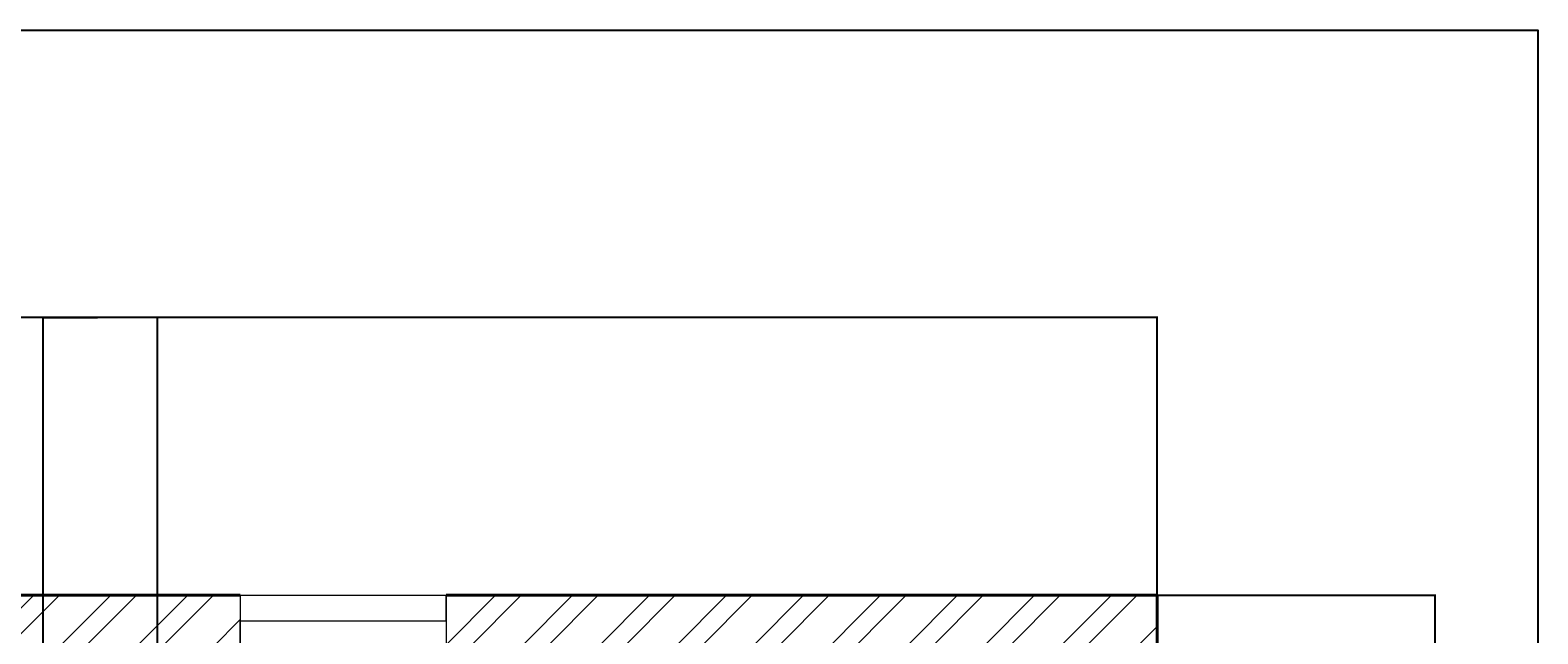
# Model space of a CAD drawing. Units: inches. Extents: x 1601 to 2297, y 1496 to 2631.
# Tile 57 of 57: x 2033 to 2297, y 2526 to 2631. Entities that reach past the tile are written whole.
import ezdxf

# ---------------------------------------------------------------- set-up
doc = ezdxf.new("R2010")
doc.units = ezdxf.units.IN
for name, color, linetype, lineweight in [('A-ANNO-DIMS', 2, 'Continuous', 18), ('A-ANNO-TTLB', 7, 'Continuous', 25), ('A-GLAZ', 161, 'Continuous', 20), ('A-WALL', 7, 'Continuous', 40), ('A-WALL-PATT', 215, 'Continuous', 13)]:
    doc.layers.add(name, color=color, linetype=linetype, lineweight=lineweight)
doc.styles.get("Standard").update_dxf_attribs({"font": 'arial.ttf'})
doc.dimstyles.get("Standard").update_dxf_attribs({"dimtxt": 0.18, "dimasz": 0.18, "dimexe": 0.18, "dimexo": 0.0625, "dimgap": 0.09, "dimtad": 0, "dimtih": 1, "dimtoh": 1, "dimdec": 4, "dimzin": 0, "dimdsep": 46, "dimtxsty": 'Standard', "dimcen": 0.09, "dimadec": 0, "dimazin": 0, "dimtfac": 1, "dimtdec": 4, "dimtofl": 0, "dimtmove": 0, "dimatfit": 3, "dimfxl": 1, "dimtolj": 1, "dimtzin": 0, "dimarcsym": 0})

# ---------------------------------------------------------------- blocks, each defined once
blk = doc.blocks.new('*D28')
at = {"layer": 'A-ANNO-DIMS', "color": 0, "lineweight": -2, "transparency": 16777216}
for p, q in [((1686.04, 2532.39), (1686.04, 2581.06)), ((1686.22, 2580.88), (1957.89, 2580.88)), ((2230.36, 2580.88), (1958.68, 2580.88)), ((2230.54, 2532.39), (2230.54, 2581.06))]:
    blk.add_line(p, q, dxfattribs=at)
at = {"layer": 'A-ANNO-DIMS', "color": 0, "transparency": 16777216}
for points in [[(1686.22, 2580.91), (1686.22, 2580.85), (1686.04, 2580.88)], [(2230.36, 2580.91), (2230.36, 2580.85), (2230.54, 2580.88)]]:
    blk.add_solid(points, dxfattribs=at)
at = {"layer": 'Defpoints', "color": 0, "transparency": 16777216}
for p in [(2230.54, 2580.88), (1686.04, 2532.33), (2230.54, 2532.33)]:
    blk.add_point(p, dxfattribs=at)
at = {"layer": 'A-ANNO-DIMS', "color": 0, "transparency": 16777216, "insert": (1958.29, 2580.88), "char_height": 0.18, "attachment_point": 5}
blk.add_mtext('\\A1;544.5', dxfattribs=at)
blk = doc.blocks.new('*D29')
at = {"layer": 'A-ANNO-DIMS', "color": 0, "lineweight": -2, "transparency": 16777216}
for p, q in [((2230.6, 2532.33), (2279.27, 2532.33)), ((2279.09, 2532.15), (2279.09, 2084.01)), ((2279.09, 1635.51), (2279.09, 2083.64)), ((2230.6, 1635.33), (2279.27, 1635.33))]:
    blk.add_line(p, q, dxfattribs=at)
at = {"layer": 'A-ANNO-DIMS', "color": 0, "transparency": 16777216}
for points in [[(2279.06, 2532.15), (2279.12, 2532.15), (2279.09, 2532.33)], [(2279.06, 1635.51), (2279.12, 1635.51), (2279.09, 1635.33)]]:
    blk.add_solid(points, dxfattribs=at)
at = {"layer": 'Defpoints', "color": 0, "transparency": 16777216}
for p in [(2230.54, 2532.33), (2279.09, 2532.33), (2230.54, 1635.33)]:
    blk.add_point(p, dxfattribs=at)
at = {"layer": 'A-ANNO-DIMS', "color": 0, "transparency": 16777216, "insert": (2279.09, 2083.83), "char_height": 0.18, "attachment_point": 5}
blk.add_mtext('\\A1;897', dxfattribs=at)
blk = doc.blocks.new('*D40')
at = {"layer": 'A-ANNO-DIMS', "color": 0, "lineweight": -2, "transparency": 16777216}
for p, q in [((2035.54, 1986.39), (2035.54, 2581.06)), ((2035.72, 2580.88), (2045.08, 2580.88)), ((2055.37, 2580.88), (2046.01, 2580.88)), ((2055.55, 1986.39), (2055.55, 2581.06))]:
    blk.add_line(p, q, dxfattribs=at)
at = {"layer": 'A-ANNO-DIMS', "color": 0, "transparency": 16777216}
for points in [[(2035.72, 2580.91), (2035.72, 2580.85), (2035.54, 2580.88)], [(2055.37, 2580.91), (2055.37, 2580.85), (2055.55, 2580.88)]]:
    blk.add_solid(points, dxfattribs=at)
at = {"layer": 'Defpoints', "color": 0, "transparency": 16777216}
for p in [(2055.55, 2580.88), (2035.54, 1986.33), (2055.55, 1986.33)]:
    blk.add_point(p, dxfattribs=at)
at = {"layer": 'A-ANNO-DIMS', "color": 0, "transparency": 16777216, "insert": (2045.54, 2580.88), "char_height": 0.18, "attachment_point": 5}
blk.add_mtext('\\A1;20.014', dxfattribs=at)

msp = doc.modelspace()

# ---------------------------------------------------------------- hatches: boundary and pattern name
at = {"layer": 'A-WALL-PATT'}
h = msp.add_hatch(dxfattribs=at)
h.set_pattern_fill('ANSI32', color=256)
h.paths.add_polyline_path([(2230.5373, 2532.3254), (2106.0595, 2532.3254), (2106.0595, 2523.3254), (2169.0373, 2523.3254), (2169.0373, 2424.3254), (2091.3989, 2424.3254), (2091.3989, 2419.8254), (2169.0373, 2419.8254), (2169.0373, 2408.1385), (2178.0373, 2408.1385), (2178.0373, 2419.8254), (2181.0581, 2419.8254), (2181.0581, 2422.0754), (2181.0581, 2424.3254), (2178.0373, 2424.3254), (2178.0373, 2523.3254), (2226.0373, 2523.3254), (2226.0373, 2424.3254), (2206.6251, 2424.3254), (2206.6251, 2419.8254), (2226.0373, 2419.8254), (2226.0373, 2299.8254), (2226.0373, 2295.3254), (2178.0373, 2295.3254), (2178.0373, 2312.1385), (2169.0373, 2312.1385), (2169.0373, 2295.3254), (2130.0373, 2295.3254), (2130.0373, 2279.1364), (2128.0593, 2279.1364), (2128.0593, 2274.6364), (2130.0373, 2274.6364), (2130.0373, 2260.7505), (2134.5373, 2260.7505), (2134.5373, 2290.8254), (2226.0373, 2290.8254), (2226.0373, 2279.2475), (2230.5373, 2279.2475), (2230.5373, 2347.8254)])
h.paths.add_polyline_path([(2070.0595, 2532.3254), (2031.0373, 2532.3254), (2031.0373, 2466.3254), (2003.9878, 2466.3254), (2003.9878, 2457.3254), (2031.0373, 2457.3254), (2031.0373, 2419.8254), (2031.0373, 2373.1914), (2035.5373, 2373.1914), (2035.5373, 2419.8254), (2047.3393, 2419.8254), (2047.3393, 2424.3254), (2035.5373, 2424.3254), (2035.5373, 2523.3254), (2070.0595, 2523.3254), (2070.0595, 2527.8254)])
h.paths.add_polyline_path([(1893.0373, 2532.3254), (1866.0336, 2532.3254), (1866.0336, 2523.3254), (1888.5373, 2523.3254), (1888.5373, 2347.8254), (1893.0373, 2347.8254), (1893.0373, 2457.3254), (1907.9878, 2457.3254), (1907.9878, 2466.3254), (1893.0373, 2466.3254)])

# ---------------------------------------------------------------- linework, layer by layer
at = {"layer": 'A-ANNO-TTLB'}
msp.add_lwpolyline([(1600.5933, 2631.1477), (2297.129, 2631.1477), (2297.129, 1496.1026), (1600.5933, 1496.1026)], close=True, dxfattribs=at)
at = {"layer": 'A-GLAZ'}
for p, q in [((2070.0595, 2532.3254), (2070.0595, 2523.3254)), ((2070.0595, 2532.3254), (2106.0595, 2532.3254)), ((2106.0595, 2527.8254), (2106.0595, 2532.3254)), ((2106.0595, 2532.3254), (2106.0595, 2532.3254)), ((2106.0595, 2532.3254), (2106.0595, 2523.3254)), ((2070.0595, 2523.3254), (2070.0595, 2527.8254)), ((2070.0595, 2527.8254), (2106.0595, 2527.8254))]:
    msp.add_line(p, q, dxfattribs=at)
at = {"layer": 'A-WALL'}
for p, q in [((1866.0336, 2532.3254), (2070.0595, 2532.3254)), ((2106.0595, 2532.3254), (2230.5373, 2532.3254)), ((2230.5373, 2532.3254), (2230.5373, 2347.8254))]:
    msp.add_line(p, q, dxfattribs=at)

# ---------------------------------------------------------------- dimensions: what is measured, and where the dimension line sits
at = {"layer": 'A-ANNO-DIMS'}
for base, p1, p2, override, picture, middle in [((2230.5373, 2580.8754), (1686.0373, 2532.3254), (2230.5373, 2532.3254), {"dimdec": 1, "dimlfac": 1, "dimrnd": 0, "dimzin": 0, "dimdsep": 46, "dimlunit": 2}, '*D28', (1958.2873, 2580.8754)), ((2055.5513, 2580.8754), (2035.5373, 1986.3254), (2055.5513, 1986.3254), {"dimdec": 3, "dimlfac": 1, "dimrnd": 0, "dimzin": 0, "dimdsep": 46, "dimlunit": 2}, '*D40', (2045.5443, 2580.8754))]:
    dim = msp.add_linear_dim(base=base, p1=p1, p2=p2, dimstyle='Standard', override=override, dxfattribs=at)
    dim.commit()
    dim.dimension.update_dxf_attribs({"geometry": picture, "text_midpoint": middle})
dim = msp.add_linear_dim(base=(2279.0873, 2532.3254), p1=(2230.5373, 1635.3254), p2=(2230.5373, 2532.3254), angle=90, dimstyle='Standard', override={"dimdec": 0, "dimlfac": 1, "dimrnd": 0, "dimzin": 0, "dimdsep": 46, "dimlunit": 2}, dxfattribs=at)
dim.commit()
dim.dimension.update_dxf_attribs({"geometry": '*D29', "text_midpoint": (2279.0873, 2083.8254)})

doc.saveas('drawing.dxf')
